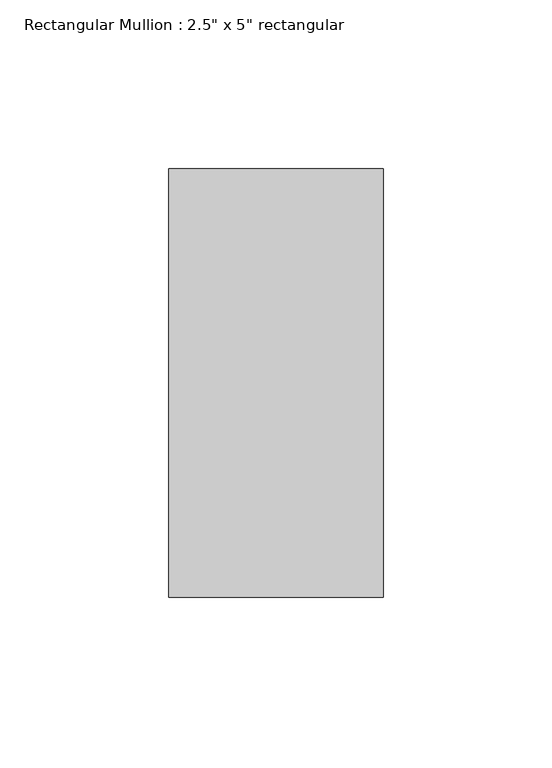
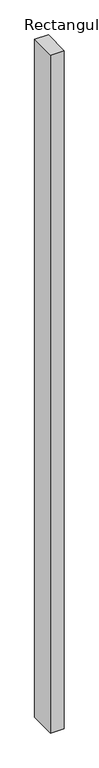
"""IFC4 building model written with IfcOpenShell, lengths in millimetres: member geometry."""

from ifc_helpers import new_model, si_unit, frame, origin, place, context, project, spatial, polyline, outline, extrude, source, transform, mapped, element, save


def member_085be126(model_context):
    return source(origin(), model_context, "Body", "SweptSolid", [
        extrude(outline(polyline([(0.0, 63.5), (0.0, -63.5), (-63.5, -63.5), (-63.5, 63.5), (0.0, 63.5)])), frame((0.0, 0.0, -3340.6541927), z_axis=(0.0, 0.0, 1.0), x_axis=(1.0, 0.0, 0.0)), (0.0, 0.0, 1.0), 3340.6541927),
    ])


if __name__ == "__main__":
    model = new_model("IFC4")
    model_context = context("Model", 3, world=origin())
    ifc_project = project(units=[si_unit("LENGTHUNIT", "METRE", prefix="MILLI")], contexts=[model_context])
    site = spatial("IfcSite", under=ifc_project)
    building = spatial("IfcBuilding", under=site)
    placement = place(None, origin())
    member_shape = member_085be126(model_context)
    element("IfcMember", 1, ObjectType="Rectangular Mullion : 2.5\" x 5\" rectangular", at=placement, inside=building, context=model_context, shape_type="MappedRepresentation", body=[
        mapped(member_shape, transform((0.0, 0.0, 0.0), x_axis=(1.0, 0.0, 0.0), y_axis=(0.0, 1.0, 0.0), z_axis=(0.0, 0.0, 1.0))),
    ])
    save(model, "model.ifc")

# Revit data of these elements
# Type "Rectangular Mullion : 2.5\" x 5\" rectangular"
#   built-in parameter 1007304 = 0.416667 (stored number, unit not read)
#   built-in parameter 1007301 = 0.104167 (stored number, unit not read)
#   built-in parameter 1007300 = 0.104167 (stored number, unit not read)
# Element 1 (IfcMember, "Rectangular Mullion : 2.5\" x 5\" rectangular")
#   Materials on its faces: "Aluminum"
# Materials
#   "Aluminum": class "Metal", colour RGB 247 247 247, transparency 0, Description = "Aluminum 6061", Cost = 0
